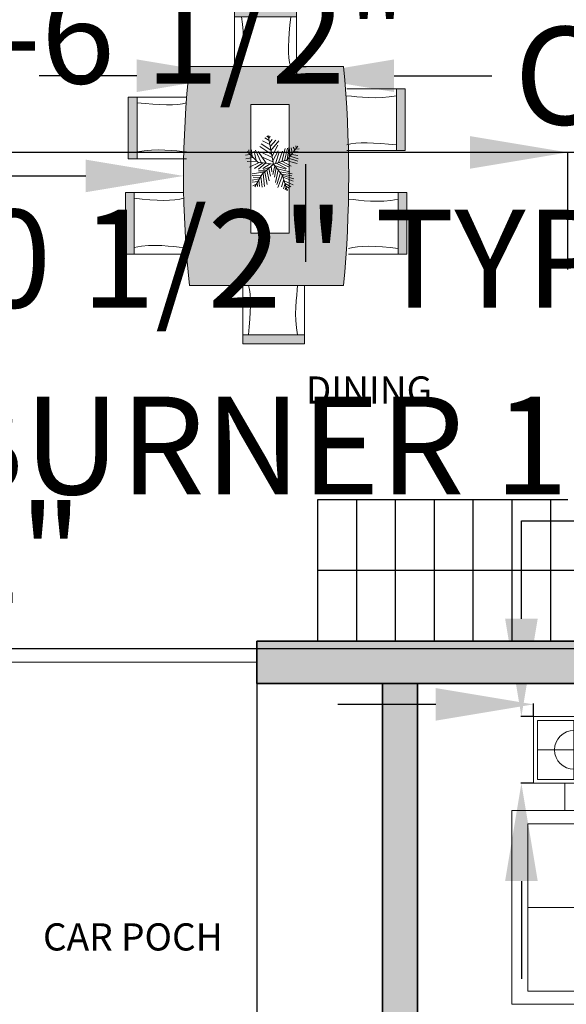
# Model space of a CAD drawing. Units: inches. Extents: x 29 to 6336, y 3 to 2592.
# Tile 5 of 8: x 5531 to 5672, y 2100 to 2354. Entities that reach past the tile are written whole.
import ezdxf

# ---------------------------------------------------------------- set-up
doc = ezdxf.new("R2010")
doc.units = ezdxf.units.IN
doc.header["$MEASUREMENT"] = 0
for name, color, linetype, lineweight in [('A-ANNO-DIMS', 2, 'Continuous', 18), ('A-AREA-IDEN', 7, 'Continuous', 18), ('A-DOOR', 4, 'Continuous', 18), ('A-FLOR-PATT', 9, 'Continuous', 13), ('A-FLOR-STRS', 7, 'Continuous', 25), ('A-FURN', 8, 'Continuous', 18), ('A-FURN-PATT', 18, 'Continuous', 13), ('A-WALL', 7, 'Continuous', 35), ('A-WALL-PATT', 242, 'Continuous', 13), ('L-PLNT', 94, 'Continuous', 18)]:
    doc.layers.add(name, color=color, linetype=linetype, lineweight=lineweight)
doc.styles.get("Standard").update_dxf_attribs({"font": 'arial.ttf'})
doc.dimstyles.get("Standard").update_dxf_attribs({"dimtxt": 25.18, "dimasz": 25.18, "dimexe": 0.18, "dimexo": 0.0625, "dimgap": 0.09, "dimtad": 0, "dimtih": 1, "dimtoh": 1, "dimdec": 0, "dimzin": 0, "dimdsep": 46, "dimlunit": 3, "dimtxsty": 'Standard', "dimcen": 0.09, "dimadec": 0, "dimazin": 0, "dimtfac": 1, "dimtdec": 0, "dimtofl": 0, "dimtmove": 0, "dimatfit": 3, "dimfxl": 1, "dimtolj": 1, "dimtzin": 0, "dimarcsym": 0})

# ---------------------------------------------------------------- blocks, each defined once
blk = doc.blocks.new('*U2')
for p, q in [((-5.114, 28.097), (-24.676, 40.636)), ((-7.288, 39.707), (-21.778, 46.673)), ((-8.737, 47.138), (-17.069, 52.711)), ((-10.186, 53.64), (-13.084, 55.962)), ((0, 0), (-10.5, 57)), ((-9.099, 51.782), (-6.563, 55.962)), ((-7.65, 43.423), (-2.578, 49.46)), ((-5.839, 35.992), (4.667, 48.067)), ((-5.114, 27.632), (10.463, 46.673)), ((-47.498, 19.737), (-55.83, 18.344)), ((-31.5, 4.5), (-52.5, 25.5)), ((-48.585, 21.131), (-49.309, 29.026)), ((-43.513, 28.561), (-42.427, 15.558)), ((-38.442, 26.239), (-34.819, 7.663)), ((-35.544, 28.097), (-24.314, 3.947)), ((-14.533, 2.09), (-30.834, 25.31)), ((-3.665, 19.273), (-27.574, 35.527)), ((-24.314, 23.917), (-2.941, 13.7)), ((-2.941, 16.486), (8.652, 37.85)), ((-1.129, 6.734), (9.014, 26.704)), ((3.942, 1.625), (11.187, 24.381)), ((10.101, 3.483), (17.708, 26.239)), ((16.259, 5.805), (23.142, 31.348)), ((22.055, 7.198), (27.489, 32.277)), ((27, 9), (48, 36)), ((27.127, 9.056), (31.112, 35.992)), ((31.836, 30.883), (32.561, 16.486)), ((35.096, 32.741), (37.27, 22.524)), ((36.183, 19.737), (48.137, 17.88)), ((38.719, 34.134), (41.979, 28.561)), ((40.53, 25.775), (48.862, 24.846)), ((43.791, 29.954), (51.036, 30.883)), ((44.153, 36.456), (45.239, 32.741)), ((-40.615, 13.7), (-55.105, 10.913)), ((-33.37, 6.269), (-52.207, 5.34)), ((-28.299, 3.483), (-47.86, -5.805)), ((-21.416, 3.018), (-38.079, -8.128)), ((0, 0), (-31.5, 4.5)), ((-15.982, 2.09), (-30.11, -9.521)), ((0, 0), (-22.5, -19.5)), ((-6.563, 1.161), (-21.416, -8.128)), ((-20.691, 13.7), (-1.129, 4.876)), ((0, 0), (27, 9)), ((0, 0), (18, -22.5)), ((6.478, 1.625), (26.04, -8.592)), ((11.187, 3.483), (30.749, -5.805)), ((18.07, 5.805), (35.096, -3.483)), ((24.229, 7.663), (46.688, 1.625)), ((29.662, 12.307), (48.137, 6.269)), ((33.285, 16.486), (48.862, 10.913)), ((-17.431, -15.094), (-42.789, -18.809)), ((-22.5, -19.5), (-37.5, -45)), ((-15.257, -12.772), (-30.11, -12.772)), ((-20.691, -18.345), (-17.793, -44.352)), ((-6.563, -5.805), (-19.967, -9.985)), ((-17.069, -15.094), (-12.721, -40.172)), ((-13.446, -11.378), (-8.737, -32.741)), ((-9.461, -8.592), (-6.201, -23.453)), ((-4.752, -3.483), (-3.665, -14.629)), ((2.493, -3.019), (-1.491, -20.202)), ((1.769, -2.555), (24.229, -9.521)), ((5.029, -6.27), (2.131, -25.775)), ((9.014, -11.378), (3.58, -35.992)), ((14.085, -16.951), (6.478, -40.172)), ((7.565, -9.056), (32.198, -14.629)), ((12.274, -15.094), (36.907, -18.809)), ((-28.299, -29.026), (-42.789, -31.348)), ((-24.314, -21.596), (-42.427, -22.06)), ((-30.834, -34.135), (-42.427, -35.528)), ((-26.849, -26.24), (-40.253, -25.775)), ((-32.646, -36.921), (-31.921, -44.352)), ((-29.023, -30.884), (-27.936, -43.887)), ((-25.038, -23.918), (-22.865, -45.281)), ((18.07, -22.524), (8.289, -45.745)), ((20.244, -30.419), (15.897, -44.816)), ((16.259, -19.738), (36.183, -22.989)), ((18, -22.5), (27, -52.5)), ((18.433, -22.524), (40.53, -29.026)), ((19.157, -25.311), (38.719, -33.206)), ((22.78, -37.85), (19.519, -48.532)), ((21.331, -32.741), (39.081, -40.636)), ((22.78, -38.314), (34.372, -44.816)), ((-34.457, -39.708), (-40.978, -42.494)), ((24.591, -45.745), (23.142, -50.854)), ((24.591, -43.423), (30.749, -47.603)), ((26.764, -49.925), (28.213, -50.854))]:
    blk.add_line(p, q)
blk = doc.blocks.new('CHAIR-DINING')
h = blk.add_hatch(color=256)
h.dxf.hatch_style = 1
h.paths.add_polyline_path([(15.9, 12.75), (15.9, 15.02), (0, 15.02), (0, 12.75)])
for p, q in [((0, 0), (0, 15.02)), ((0, 15.02), (15.9, 15.02)), ((0, 12.75), (15.9, 12.75)), ((15.9, 15.02), (15.9, 0))]:
    blk.add_line(p, q)
for points in [[(1.75, 12.75), (2.84, 7.81), (1.97, 2.88), (1.75, 0)], [(14.44, 12.75), (13.78, 7.03), (13.63, 2.52), (14.44, 0)]]:
    blk.add_open_spline(points, degree=3)
blk = doc.blocks.new('SOFA-TWO-SEAT')
blk.add_line((4.12, 24.97), (26.62, 24.97))
for points in [[(4.17, 49.94), (0, 49.94), (0, 0), (4.17, 0)], [(4.17, 49.94), (26.62, 49.94), (26.62, 46.51), (4.17, 46.51)], [(4.17, 3.43), (4.17, 46.51)], [(4.12, 3.43), (26.57, 3.43), (26.57, 0), (4.12, 0)]]:
    blk.add_lwpolyline(points)
blk.add_lwpolyline([(26.62, 46.51), (4.12, 46.51), (4.12, 3.43), (26.62, 3.43)], close=True)
blk = doc.blocks.new('END-TABLE-21X17')
for p, q in [((10.41, 16.21), (10.41, 1)), ((1, 8.6), (19.81, 8.6))]:
    blk.add_line(p, q)
for points in [[(0, 17.21), (20.81, 17.21), (20.81, 0), (0, 0)], [(1, 16.21), (19.81, 16.21), (19.81, 1), (1, 1)]]:
    blk.add_lwpolyline(points, close=True)
blk.add_circle((10.41, 8.6), 5)
blk = doc.blocks.new('*D20')
at = {"layer": 'A-ANNO-DIMS', "color": 0, "lineweight": -2, "transparency": 16777216}
for p, q in [((5586.64, 2341.55), (5586.64, 2339.04)), ((5602.54, 2341.55), (5602.54, 2339.04)), ((5561.46, 2339.22), (5536.28, 2339.22)), ((5627.72, 2339.22), (5652.9, 2339.22))]:
    blk.add_line(p, q, dxfattribs=at)
at = {"layer": 'A-ANNO-DIMS', "color": 0, "transparency": 16777216}
for points in [[(5561.46, 2343.42), (5561.46, 2335.03), (5586.64, 2339.22)], [(5627.72, 2343.42), (5627.72, 2335.03), (5602.54, 2339.22)]]:
    blk.add_solid(points, dxfattribs=at)
at = {"layer": 'Defpoints', "color": 0, "transparency": 16777216}
for p in [(5586.64, 2341.61), (5602.54, 2341.61), (5602.54, 2339.22)]:
    blk.add_point(p, dxfattribs=at)
at = {"layer": 'A-ANNO-DIMS', "color": 0, "transparency": 16777216, "insert": (5789.2, 2339.22), "char_height": 25.18, "attachment_point": 5}
blk.add_mtext('\\A1;CHAIR 1\'-4" TYP.', dxfattribs=at)
blk = doc.blocks.new('*D21')
at = {"layer": 'A-ANNO-DIMS', "color": 0, "lineweight": -2, "transparency": 16777216}
for p, q in [((5604.93, 2381.81), (5604.93, 2406.99)), ((5604.93, 2406.99), (5630.11, 2406.99)), ((5602.6, 2356.63), (5605.11, 2356.63)), ((5602.6, 2341.61), (5605.11, 2341.61)), ((5604.93, 2316.43), (5604.93, 2291.25))]:
    blk.add_line(p, q, dxfattribs=at)
at = {"layer": 'A-ANNO-DIMS', "color": 0, "transparency": 16777216}
for points in [[(5600.73, 2381.81), (5609.12, 2381.81), (5604.93, 2356.63)], [(5600.73, 2316.43), (5609.12, 2316.43), (5604.93, 2341.61)]]:
    blk.add_solid(points, dxfattribs=at)
at = {"layer": 'Defpoints', "color": 0, "transparency": 16777216}
for p in [(5602.54, 2356.63), (5604.93, 2356.63), (5602.54, 2341.61)]:
    blk.add_point(p, dxfattribs=at)
at = {"layer": 'A-ANNO-DIMS', "color": 0, "transparency": 16777216, "insert": (5705.75, 2406.99), "char_height": 25.18, "attachment_point": 5}
blk.add_mtext('\\A1;1\'-3" TYP.', dxfattribs=at)
blk = doc.blocks.new('*D24')
at = {"layer": 'A-ANNO-DIMS', "color": 0, "lineweight": -2, "transparency": 16777216}
for p, q in [((5412.73, 2243.97), (5387.55, 2243.97)), ((5437.91, 2241.81), (5437.91, 2244.15)), ((5452.73, 2241.81), (5452.73, 2244.15)), ((5477.91, 2243.97), (5503.09, 2243.97))]:
    blk.add_line(p, q, dxfattribs=at)
at = {"layer": 'A-ANNO-DIMS', "color": 0, "transparency": 16777216}
for points in [[(5412.73, 2248.16), (5412.73, 2239.77), (5437.91, 2243.97)], [(5477.91, 2248.16), (5477.91, 2239.77), (5452.73, 2243.97)]]:
    blk.add_solid(points, dxfattribs=at)
at = {"layer": 'Defpoints', "color": 0, "transparency": 16777216}
for p in [(5452.73, 2243.97), (5437.91, 2241.74), (5452.73, 2241.74)]:
    blk.add_point(p, dxfattribs=at)
at = {"layer": 'A-ANNO-DIMS', "color": 0, "transparency": 16777216, "insert": (5658.52, 2243.97), "char_height": 25.18, "attachment_point": 5}
blk.add_mtext('\\A1;BURNER 1\'-3" TYP.', dxfattribs=at)
blk = doc.blocks.new('*D25')
at = {"layer": 'A-ANNO-DIMS', "color": 0, "lineweight": -2, "transparency": 16777216}
for p, q in [((5435.68, 2266.92), (5435.68, 2292.1)), ((5435.68, 2292.1), (5460.86, 2292.1)), ((5437.84, 2241.74), (5435.5, 2241.74)), ((5437.84, 2231.12), (5435.5, 2231.12)), ((5435.68, 2205.94), (5435.68, 2180.76))]:
    blk.add_line(p, q, dxfattribs=at)
at = {"layer": 'A-ANNO-DIMS', "color": 0, "transparency": 16777216}
for points in [[(5431.49, 2266.92), (5439.88, 2266.92), (5435.68, 2241.74)], [(5431.49, 2205.94), (5439.88, 2205.94), (5435.68, 2231.12)]]:
    blk.add_solid(points, dxfattribs=at)
at = {"layer": 'Defpoints', "color": 0, "transparency": 16777216}
for p in [(5435.68, 2241.74), (5437.91, 2241.74), (5437.91, 2231.12)]:
    blk.add_point(p, dxfattribs=at)
at = {"layer": 'A-ANNO-DIMS', "color": 0, "transparency": 16777216, "insert": (5576.81, 2292.1), "char_height": 25.18, "attachment_point": 5}
blk.add_mtext('\\A1;0\'-10 1/2" TYP.', dxfattribs=at)
blk = doc.blocks.new('*D28')
at = {"layer": 'A-ANNO-DIMS', "color": 0, "lineweight": -2, "transparency": 16777216}
for p, q in [((5689.81, 2064.89), (5689.81, 2057.28)), ((5739.75, 2064.89), (5739.75, 2057.28)), ((5664.63, 2057.46), (5639.45, 2057.46)), ((5764.93, 2057.46), (5790.11, 2057.46))]:
    blk.add_line(p, q, dxfattribs=at)
at = {"layer": 'A-ANNO-DIMS', "color": 0, "transparency": 16777216}
for points in [[(5664.63, 2061.65), (5664.63, 2053.26), (5689.81, 2057.46)], [(5764.93, 2061.65), (5764.93, 2053.26), (5739.75, 2057.46)]]:
    blk.add_solid(points, dxfattribs=at)
at = {"layer": 'Defpoints', "color": 0, "transparency": 16777216}
for p in [(5689.81, 2064.95), (5739.75, 2064.95), (5689.81, 2057.46)]:
    blk.add_point(p, dxfattribs=at)
at = {"layer": 'A-ANNO-DIMS', "color": 0, "transparency": 16777216, "insert": (5509.91, 2057.46), "char_height": 25.18, "attachment_point": 5}
blk.add_mtext('\\A1;SOFA 4\'-2" TYP.', dxfattribs=at)
blk = doc.blocks.new('*D29')
at = {"layer": 'A-ANNO-DIMS', "color": 0, "lineweight": -2, "transparency": 16777216}
for p, q in [((5682.32, 2116.75), (5682.32, 2141.93)), ((5689.75, 2091.57), (5682.14, 2091.57)), ((5689.75, 2064.95), (5682.14, 2064.95)), ((5682.32, 2039.77), (5682.32, 2014.59))]:
    blk.add_line(p, q, dxfattribs=at)
at = {"layer": 'A-ANNO-DIMS', "color": 0, "transparency": 16777216}
for points in [[(5678.12, 2116.75), (5686.52, 2116.75), (5682.32, 2091.57)], [(5678.12, 2039.77), (5686.52, 2039.77), (5682.32, 2064.95)]]:
    blk.add_solid(points, dxfattribs=at)
at = {"layer": 'Defpoints', "color": 0, "transparency": 16777216}
for p in [(5682.32, 2091.57), (5689.81, 2091.57), (5689.81, 2064.95)]:
    blk.add_point(p, dxfattribs=at)
at = {"layer": 'A-ANNO-DIMS', "color": 0, "transparency": 16777216, "insert": (5682.32, 2078.26), "char_height": 25.18, "attachment_point": 5}
blk.add_mtext('\\A1;2\'-2 1/2" TYP.', dxfattribs=at)
blk = doc.blocks.new('*D34')
at = {"layer": 'A-ANNO-DIMS', "color": 0, "lineweight": -2, "transparency": 16777216}
for p, q in [((5638.44, 2177.3), (5613.26, 2177.3)), ((5663.62, 2174.24), (5663.62, 2177.48)), ((5684.43, 2174.24), (5684.43, 2177.48)), ((5709.61, 2177.3), (5734.79, 2177.3))]:
    blk.add_line(p, q, dxfattribs=at)
at = {"layer": 'A-ANNO-DIMS', "color": 0, "transparency": 16777216}
for points in [[(5638.44, 2181.49), (5638.44, 2173.1), (5663.62, 2177.3)], [(5709.61, 2181.49), (5709.61, 2173.1), (5684.43, 2177.3)]]:
    blk.add_solid(points, dxfattribs=at)
at = {"layer": 'Defpoints', "color": 0, "transparency": 16777216}
for p in [(5684.43, 2177.3), (5663.62, 2174.18), (5684.43, 2174.18)]:
    blk.add_point(p, dxfattribs=at)
at = {"layer": 'A-ANNO-DIMS', "color": 0, "transparency": 16777216, "insert": (5913.59, 2177.3), "char_height": 25.18, "attachment_point": 5}
blk.add_mtext('\\A1;END TABLE 1\'-9" TYP.', dxfattribs=at)
blk = doc.blocks.new('*D35')
at = {"layer": 'A-ANNO-DIMS', "color": 0, "lineweight": -2, "transparency": 16777216}
for p, q in [((5660.5, 2199.36), (5660.5, 2224.54)), ((5660.5, 2224.54), (5685.68, 2224.54)), ((5663.56, 2174.18), (5660.32, 2174.18)), ((5663.56, 2156.97), (5660.32, 2156.97)), ((5660.5, 2131.79), (5660.5, 2106.61))]:
    blk.add_line(p, q, dxfattribs=at)
at = {"layer": 'A-ANNO-DIMS', "color": 0, "transparency": 16777216}
for points in [[(5656.3, 2199.36), (5664.7, 2199.36), (5660.5, 2174.18)], [(5656.3, 2131.79), (5664.7, 2131.79), (5660.5, 2156.97)]]:
    blk.add_solid(points, dxfattribs=at)
at = {"layer": 'Defpoints', "color": 0, "transparency": 16777216}
for p in [(5660.5, 2174.18), (5663.62, 2174.18), (5663.62, 2156.97)]:
    blk.add_point(p, dxfattribs=at)
at = {"layer": 'A-ANNO-DIMS', "color": 0, "transparency": 16777216, "insert": (5761.33, 2224.54), "char_height": 25.18, "attachment_point": 5}
blk.add_mtext('\\A1;1\'-5" TYP.', dxfattribs=at)
blk = doc.blocks.new('*D39')
at = {"layer": 'A-ANNO-DIMS', "color": 0, "lineweight": -2, "transparency": 16777216}
for p, q in [((5417.07, 2045.77), (5417.07, 2070.95)), ((5417.07, 2070.95), (5442.25, 2070.95)), ((5416.29, 2020.59), (5417.25, 2020.59)), ((5416.29, 2015.87), (5417.25, 2015.87)), ((5417.07, 1990.69), (5417.07, 1965.51))]:
    blk.add_line(p, q, dxfattribs=at)
at = {"layer": 'A-ANNO-DIMS', "color": 0, "transparency": 16777216}
for points in [[(5412.88, 2045.77), (5421.27, 2045.77), (5417.07, 2020.59)], [(5412.88, 1990.69), (5421.27, 1990.69), (5417.07, 2015.87)]]:
    blk.add_solid(points, dxfattribs=at)
at = {"layer": 'Defpoints', "color": 0, "transparency": 16777216}
for p in [(5416.23, 2020.59), (5417.07, 2020.59), (5416.23, 2015.87)]:
    blk.add_point(p, dxfattribs=at)
at = {"layer": 'A-ANNO-DIMS', "color": 0, "transparency": 16777216, "insert": (5548.42, 2070.95), "char_height": 25.18, "attachment_point": 5}
blk.add_mtext('\\A1;0\'-4 1/2" TYP.', dxfattribs=at)
blk = doc.blocks.new('*D48')
at = {"layer": 'A-ANNO-DIMS', "color": 0, "lineweight": -2, "transparency": 16777216}
for p, q in [((5351.16, 2319.63), (5351.16, 2522.76)), ((5376.34, 2522.58), (5385.42, 2522.58)), ((5410.6, 2319.63), (5410.6, 2522.76)), ((5410.6, 2522.58), (5435.78, 2522.58))]:
    blk.add_line(p, q, dxfattribs=at)
at = {"layer": 'A-ANNO-DIMS', "color": 0, "transparency": 16777216}
for points in [[(5376.34, 2526.78), (5376.34, 2518.38), (5351.16, 2522.58)], [(5385.42, 2526.78), (5385.42, 2518.38), (5410.6, 2522.58)]]:
    blk.add_solid(points, dxfattribs=at)
at = {"layer": 'Defpoints', "color": 0, "transparency": 16777216}
for p in [(5410.6, 2522.58), (5351.16, 2319.56), (5410.6, 2319.56)]:
    blk.add_point(p, dxfattribs=at)
at = {"layer": 'A-ANNO-DIMS', "color": 0, "transparency": 16777216, "insert": (5508.96, 2522.58), "char_height": 25.18, "attachment_point": 5}
blk.add_mtext('\\A1;4\'-11 1/2"', dxfattribs=at)
blk = doc.blocks.new('*D49')
at = {"layer": 'A-ANNO-DIMS', "color": 0, "lineweight": -2, "transparency": 16777216}
for p, q in [((5419.6, 2191.59), (5419.6, 1921.9)), ((5510.11, 2191.59), (5510.11, 1921.9)), ((5444.78, 1922.08), (5484.93, 1922.08)), ((5510.11, 1922.08), (5535.29, 1922.08))]:
    blk.add_line(p, q, dxfattribs=at)
at = {"layer": 'A-ANNO-DIMS', "color": 0, "transparency": 16777216}
for points in [[(5444.78, 1926.28), (5444.78, 1917.88), (5419.6, 1922.08)], [(5484.93, 1926.28), (5484.93, 1917.88), (5510.11, 1922.08)]]:
    blk.add_solid(points, dxfattribs=at)
at = {"layer": 'Defpoints', "color": 0, "transparency": 16777216}
for p in [(5419.6, 2191.65), (5510.11, 2191.65), (5510.11, 1922.08)]:
    blk.add_point(p, dxfattribs=at)
at = {"layer": 'A-ANNO-DIMS', "color": 0, "transparency": 16777216, "insert": (5598.08, 1922.08), "char_height": 25.18, "attachment_point": 5}
blk.add_mtext('\\A1;7\'-6 1/2"', dxfattribs=at)
blk = doc.blocks.new('*D50')
at = {"layer": 'A-ANNO-DIMS', "color": 0, "lineweight": -2, "transparency": 16777216}
for p, q in [((5510.17, 2319.56), (5917.09, 2319.56)), ((5916.91, 2294.38), (5916.91, 2268.55)), ((5916.91, 2216.83), (5916.91, 2242.66)), ((5510.17, 2191.65), (5917.09, 2191.65))]:
    blk.add_line(p, q, dxfattribs=at)
at = {"layer": 'A-ANNO-DIMS', "color": 0, "transparency": 16777216}
for points in [[(5912.71, 2294.38), (5921.1, 2294.38), (5916.91, 2319.56)], [(5912.71, 2216.83), (5921.1, 2216.83), (5916.91, 2191.65)]]:
    blk.add_solid(points, dxfattribs=at)
at = {"layer": 'Defpoints', "color": 0, "transparency": 16777216}
for p in [(5510.11, 2319.56), (5916.91, 2319.56), (5510.11, 2191.65)]:
    blk.add_point(p, dxfattribs=at)
at = {"layer": 'A-ANNO-DIMS', "color": 0, "transparency": 16777216, "insert": (5916.91, 2255.61), "char_height": 25.18, "attachment_point": 5}
blk.add_mtext('\\A1;10\'-8"', dxfattribs=at)
blk = doc.blocks.new('*D59')
at = {"layer": 'A-ANNO-DIMS', "color": 0, "lineweight": -2, "transparency": 16777216}
for p, q in [((5519.11, 2182.59), (5519.11, 1921.9)), ((5592.36, 2182.59), (5592.36, 1921.9)), ((5493.93, 1922.08), (5468.75, 1922.08)), ((5617.54, 1922.08), (5642.72, 1922.08))]:
    blk.add_line(p, q, dxfattribs=at)
at = {"layer": 'A-ANNO-DIMS', "color": 0, "transparency": 16777216}
for points in [[(5493.93, 1926.28), (5493.93, 1917.88), (5519.11, 1922.08)], [(5617.54, 1926.28), (5617.54, 1917.88), (5592.36, 1922.08)]]:
    blk.add_solid(points, dxfattribs=at)
at = {"layer": 'Defpoints', "color": 0, "transparency": 16777216}
for p in [(5519.11, 2182.65), (5592.36, 2182.65), (5592.36, 1922.08)]:
    blk.add_point(p, dxfattribs=at)
at = {"layer": 'A-ANNO-DIMS', "color": 0, "transparency": 16777216, "insert": (5555.73, 1922.08), "char_height": 25.18, "attachment_point": 5}
blk.add_mtext('\\A1;6\'-1"', dxfattribs=at)
blk = doc.blocks.new('*D60')
at = {"layer": 'A-ANNO-DIMS', "color": 0, "lineweight": -2, "transparency": 16777216}
for p, q in [((5647.28, 2319.47), (5622.1, 2319.47)), ((5672.46, 2289.28), (5672.46, 2319.65)), ((5712.66, 2289.28), (5712.66, 2319.65)), ((5737.84, 2319.47), (5763.02, 2319.47))]:
    blk.add_line(p, q, dxfattribs=at)
at = {"layer": 'A-ANNO-DIMS', "color": 0, "transparency": 16777216}
for points in [[(5647.28, 2323.67), (5647.28, 2315.27), (5672.46, 2319.47)], [(5737.84, 2323.67), (5737.84, 2315.27), (5712.66, 2319.47)]]:
    blk.add_solid(points, dxfattribs=at)
at = {"layer": 'Defpoints', "color": 0, "transparency": 16777216}
for p in [(5712.66, 2319.47), (5672.46, 2289.22), (5712.66, 2289.22)]:
    blk.add_point(p, dxfattribs=at)
at = {"layer": 'A-ANNO-DIMS', "color": 0, "transparency": 16777216, "insert": (5796.57, 2319.47), "char_height": 25.18, "attachment_point": 5}
blk.add_mtext('\\A1;3\'-4"', dxfattribs=at)
blk = doc.blocks.new('*D68')
at = {"layer": 'A-ANNO-DIMS', "color": 0, "lineweight": -2, "transparency": 16777216}
for p, q in [((5479.86, 2259.85), (5479.86, 2285.03)), ((5510.05, 2234.67), (5479.68, 2234.67)), ((5510.05, 2197.33), (5479.68, 2197.33)), ((5479.86, 2172.15), (5479.86, 2146.97))]:
    blk.add_line(p, q, dxfattribs=at)
at = {"layer": 'A-ANNO-DIMS', "color": 0, "transparency": 16777216}
for points in [[(5475.66, 2259.85), (5484.06, 2259.85), (5479.86, 2234.67)], [(5475.66, 2172.15), (5484.06, 2172.15), (5479.86, 2197.33)]]:
    blk.add_solid(points, dxfattribs=at)
at = {"layer": 'Defpoints', "color": 0, "transparency": 16777216}
for p in [(5479.86, 2234.67), (5510.11, 2234.67), (5510.11, 2197.33)]:
    blk.add_point(p, dxfattribs=at)
at = {"layer": 'A-ANNO-DIMS', "color": 0, "transparency": 16777216, "insert": (5479.86, 2216), "char_height": 25.18, "attachment_point": 5}
blk.add_mtext('\\A1;3\'-1 1/2"', dxfattribs=at)
blk = doc.blocks.new('*D69')
at = {"layer": 'A-ANNO-DIMS', "color": 0, "lineweight": -2, "transparency": 16777216}
for p, q in [((5394.42, 2349.81), (5369.24, 2349.81)), ((5419.6, 2319.63), (5419.6, 2349.99)), ((5450.34, 2319.63), (5450.34, 2349.99)), ((5475.52, 2349.81), (5500.7, 2349.81))]:
    blk.add_line(p, q, dxfattribs=at)
at = {"layer": 'A-ANNO-DIMS', "color": 0, "transparency": 16777216}
for points in [[(5394.42, 2354.01), (5394.42, 2345.62), (5419.6, 2349.81)], [(5475.52, 2354.01), (5475.52, 2345.62), (5450.34, 2349.81)]]:
    blk.add_solid(points, dxfattribs=at)
at = {"layer": 'Defpoints', "color": 0, "transparency": 16777216}
for p in [(5450.34, 2349.81), (5419.6, 2319.56), (5450.34, 2319.56)]:
    blk.add_point(p, dxfattribs=at)
at = {"layer": 'A-ANNO-DIMS', "color": 0, "transparency": 16777216, "insert": (5563.81, 2349.81), "char_height": 25.18, "attachment_point": 5}
blk.add_mtext('\\A1;2\'-6 1/2"', dxfattribs=at)
blk = doc.blocks.new('*D71')
at = {"layer": 'A-ANNO-DIMS', "color": 0, "lineweight": -2, "transparency": 16777216}
for p, q in [((5510.6, 2313.41), (5548.31, 2313.41)), ((5835.74, 2313.41), (5835.92, 2313.41)), ((5835.83, 2313.32), (5835.83, 2313.5))]:
    blk.add_line(p, q, dxfattribs=at)
at = {"layer": 'A-ANNO-DIMS', "color": 0, "transparency": 16777216}
blk.add_solid([(5548.31, 2317.61), (5548.31, 2309.22), (5573.49, 2313.41)], dxfattribs=at)
at = {"layer": 'Defpoints', "color": 0, "transparency": 16777216}
for p in [(5573.49, 2313.41), (5835.83, 2313.41)]:
    blk.add_point(p, dxfattribs=at)
at = {"layer": 'A-ANNO-DIMS', "color": 0, "transparency": 16777216, "insert": (5416.09, 2313.41), "char_height": 25.18, "attachment_point": 5}
blk.add_mtext('\\A1;R21\'-10 1/2"', dxfattribs=at)

msp = doc.modelspace()

# ---------------------------------------------------------------- hatches: boundary and pattern name
at = {"layer": 'A-FURN-PATT'}
h = msp.add_hatch(color=256, dxfattribs=at)
h.dxf.hatch_style = 1
h.paths.add_polyline_path([(5614.72, 2341.61), (5575.01, 2341.61, 0.053894), (5575.01, 2285.22), (5614.72, 2285.22, 0.046017)])
h.paths.add_polyline_path([(5590.82, 2298.69), (5590.82, 2331.84), (5600.65, 2331.84), (5600.65, 2318.19), (5600.89, 2318.49), (5600.88, 2318.57), (5600.93, 2318.55), (5600.65, 2318.19), (5600.65, 2298.69)], flags=16)
h.paths.add_polyline_path([(5599.61, 2311.45), (5599.6, 2311.44), (5599.61, 2311.43)], flags=0)
h.paths.add_polyline_path([(5599.01, 2313.47), (5596.67, 2316.4), (5594.45, 2314.47), (5594.45, 2314.45), (5594.41, 2314.44), (5596.67, 2316.4), (5595.99, 2320.04), (5596.04, 2320.02), (5596.01, 2319.98), (5596.67, 2316.4), (5596.94, 2316.05), (5597, 2316.03), (5596.99, 2316), (5598.98, 2313.5), (5599.01, 2313.49)], flags=0)
at = {"layer": 'A-WALL-PATT'}
h = msp.add_hatch(color=256, dxfattribs=at)
h.dxf.hatch_style = 1
h.paths.add_polyline_path([(5558.68, 2492.33), (5459.71, 2492.33), (5459.71, 2483.33), (5511.77, 2483.33), (5511.77, 2388.68), (5520.77, 2388.68), (5520.77, 2393.05), (5526.31, 2393.05), (5526.31, 2402.05), (5520.77, 2402.05), (5520.77, 2483.33), (5558.68, 2483.33)])
h.paths.add_polyline_path([(5659.13, 2492.33), (5586.68, 2492.33), (5586.68, 2483.33), (5624.6, 2483.33), (5624.6, 2402.05), (5562.29, 2402.05), (5562.29, 2393.05), (5676.48, 2393.05), (5676.48, 2402.05), (5633.6, 2402.05), (5633.6, 2422.71), (5633.6, 2483.33), (5659.13, 2483.33)])
h.paths.add_polyline_path([(5886.66, 2492.33), (5687.13, 2492.33), (5687.13, 2483.33), (5712.66, 2483.33), (5712.66, 2468.69), (5721.66, 2468.69), (5721.66, 2483.33), (5877.66, 2483.33), (5877.66, 2106.48), (5858.21, 2106.48), (5858.21, 2097.48), (5877.66, 2097.48), (5877.66, 1961.33), (5877.66, 1952.33), (5886.66, 1952.33)])
h.paths.add_polyline_path([(5721.66, 2416.69), (5712.66, 2416.69), (5712.66, 2402.05), (5709.45, 2402.05), (5709.45, 2393.05), (5712.66, 2393.05), (5712.66, 2386.01), (5721.66, 2386.01)], flags=17)
h.paths.add_polyline_path([(5355.66, 2483.33), (5407.71, 2483.33), (5407.71, 2492.33), (5346.66, 2492.33), (5346.66, 2431.95), (5355.66, 2431.95)])
h.paths.add_polyline_path([(5355.66, 2379.95), (5346.66, 2379.95), (5346.66, 2319.56), (5355.66, 2319.56), (5355.66, 2328.56)])
h.paths.add_polyline_path([(5520.77, 2337.13), (5511.77, 2337.13), (5511.77, 2328.56), (5410.6, 2328.56), (5410.6, 2319.56), (5410.6, 2281.61), (5419.6, 2281.61), (5419.6, 2319.56), (5510.11, 2319.56), (5510.11, 2234.67), (5519.11, 2234.67), (5519.11, 2319.56), (5520.77, 2319.56)])
h.paths.add_polyline_path([(5519.11, 2197.33), (5510.11, 2197.33), (5510.11, 2191.65), (5419.6, 2191.65), (5419.6, 2228.6), (5419.6, 2229.61), (5410.6, 2229.61), (5410.6, 2182.65), (5519.11, 2182.65)])
h.paths.add_polyline_path([(5712.66, 2193.6), (5592.36, 2193.6), (5592.36, 2182.65), (5624.77, 2182.65), (5633.77, 2182.65), (5712.66, 2182.65)])
h.paths.add_polyline_path([(5633.77, 2182.65), (5624.77, 2182.65), (5624.77, 2051.72), (5633.77, 2051.72), (5691.77, 2051.72), (5691.77, 2060.72), (5633.77, 2060.72)])
h.paths.add_polyline_path([(5810.76, 2097.48), (5830.21, 2097.48), (5830.21, 2106.48), (5810.76, 2106.48), (5810.76, 2182.65), (5817.87, 2182.65), (5817.87, 2193.6), (5783.59, 2193.6), (5783.59, 2182.65), (5801.76, 2182.65), (5801.76, 2060.72), (5743.77, 2060.72), (5743.77, 2051.72), (5810.76, 2051.72)], flags=17)
h.paths.add_polyline_path([(5721.66, 2319.56), (5877.66, 2319.56), (5877.66, 2328.56), (5721.66, 2328.56), (5721.66, 2335.85), (5712.66, 2335.85), (5712.66, 2319.56), (5712.66, 2182.65), (5726.12, 2182.65), (5726.12, 2193.6), (5721.66, 2193.6)], flags=17)
h.paths.add_polyline_path([(5631.73, 2431.78), (5711.31, 2431.78), (5711.31, 2446.2), (5631.73, 2446.2)], flags=9)

# ---------------------------------------------------------------- linework, layer by layer
at = {"layer": 'A-DOOR'}
msp.add_line((5592.36, 2188.13), (5519.11, 2188.13), dxfattribs=at)
at = {"layer": 'A-FLOR-PATT'}
msp.add_line((5671.67, 2156.97), (5671.67, 2149.97), dxfattribs=at)
at = {"layer": 'A-FLOR-STRS'}
for p, q in [((5608.08, 2193.6), (5608.08, 2230.08)), ((5608.08, 2230.08), (5672.46, 2230.08)), ((5618.08, 2193.6), (5618.08, 2230.08)), ((5628.08, 2193.6), (5628.08, 2230.08)), ((5638.08, 2193.6), (5638.08, 2230.08)), ((5648.08, 2193.6), (5648.08, 2230.08)), ((5658.08, 2193.6), (5658.08, 2230.08)), ((5668.08, 2193.6), (5668.08, 2230.08)), ((5608.08, 2211.84), (5693.88, 2211.84))]:
    msp.add_line(p, q, dxfattribs=at)
at = {"layer": 'A-FURN'}
for points in [[(5575.01, 2341.61), (5614.72, 2341.61)], [(5614.72, 2285.22), (5614.72, 2285.22), (5575.01, 2285.22)]]:
    msp.add_lwpolyline(points, dxfattribs=at)
msp.add_lwpolyline([(5590.82, 2331.84), (5600.65, 2331.84), (5600.65, 2298.69), (5590.82, 2298.69)], close=True, dxfattribs=at)
for centre, radius, start, end in [((5835.83, 2313.41), 262.34, 173.8302, 186.1698), ((5309.02, 2313.41), 307, 354.7306, 5.2694)]:
    msp.add_arc(centre, radius, start, end, dxfattribs=at)
at = {"layer": 'A-WALL'}
for p, q in [((5592.36, 2193.6), (5712.66, 2193.6)), ((5592.36, 2193.6), (5592.36, 2182.65)), ((5592.36, 2182.65), (5624.77, 2182.65)), ((5624.77, 2182.65), (5624.77, 2051.72)), ((5624.77, 2182.65), (5633.77, 2182.65)), ((5633.77, 2182.65), (5633.77, 2060.72)), ((5633.77, 2182.65), (5712.66, 2182.65))]:
    msp.add_line(p, q, dxfattribs=at)

# ---------------------------------------------------------------- block references
at = {"layer": 'A-FURN'}
for name, p in [('CHAIR-DINING', (5586.64, 2341.61)), ('END-TABLE-21X17', (5663.62, 2156.97)), ('SOFA-TWO-SEAT', (5658, 2100.03))]:
    msp.add_blockref(name, p, dxfattribs=at)
for p, rotation in [((5574.28, 2317.84), 90.00000000001506), ((5615.57, 2335.82), 270.0000000000055), ((5573.53, 2293.22), 90.00000000000794), ((5616.01, 2309.17), 270.000000000008), ((5604.62, 2285.22), 180)]:
    msp.add_blockref('CHAIR-DINING', p, dxfattribs=dict(at, rotation=rotation))
at = {"layer": 'L-PLNT', "xscale": 0.129609211949132, "yscale": 0.129609211949132, "zscale": 0.129609211949132}
msp.add_blockref('*U2', (5596.67, 2316.4), dxfattribs=at)

# ---------------------------------------------------------------- texts
at = {"layer": 'A-AREA-IDEN', "char_height": 7, "attachment_point": 1}
for s, insert in [('DINING', (5604.97, 2261.77)), ('CAR POCH', (5537.29, 2120.89))]:
    msp.add_mtext_dynamic_manual_height_columns(s, width=54.3344, gutter_width=1, heights=[0], dxfattribs=dict(at, insert=insert))

# ---------------------------------------------------------------- dimensions: what is measured, and where the dimension line sits
at = {"layer": 'A-ANNO-DIMS'}
for base, p1, p2, picture, middle in [((5410.6, 2522.58), (5351.16, 2319.56), (5410.6, 2319.56), '*D48', (5508.96, 2522.58)), ((5450.34, 2349.81), (5419.6, 2319.56), (5450.34, 2319.56), '*D69', (5563.81, 2349.81)), ((5712.66, 2319.47), (5672.46, 2289.22), (5712.66, 2289.22), '*D60', (5796.57, 2319.47)), ((5510.11, 1922.08), (5419.6, 2191.65), (5510.11, 2191.65), '*D49', (5598.08, 1922.08)), ((5592.3592, 1922.0797), (5519.1102, 2182.6481), (5592.3592, 2182.6517), '*D59', (5555.7347, 1922.0797))]:
    dim = msp.add_linear_dim(base=base, p1=p1, p2=p2, dimstyle='Standard', override={"dimdec": 1, "dimlfac": 1, "dimrnd": 0, "dimzin": 1, "dimdsep": 46, "dimlunit": 4, "dimfrac": 2}, dxfattribs=at)
    dim.commit()
    dim.dimension.update_dxf_attribs({"geometry": picture, "text_midpoint": middle})
for base, p1, p2, angle, text, picture, middle in [((5604.93, 2356.63), (5602.54, 2341.61), (5602.54, 2356.63), 90, '<> TYP.', '*D21', (5705.75, 2406.99)), ((5435.68, 2241.74), (5437.91, 2231.12), (5437.91, 2241.74), 90, '<> TYP.', '*D25', (5576.81, 2292.1)), ((5660.5, 2174.18), (5663.62, 2156.97), (5663.62, 2174.18), 90, '<> TYP.', '*D35', (5761.33, 2224.54)), ((5682.32, 2091.57), (5689.81, 2064.95), (5689.81, 2091.57), 90, '<> TYP.', '*D29', (5682.32, 2078.26)), ((5417.07, 2020.59), (5416.23, 2015.87), (5416.23, 2020.59), 90, '<> TYP.', '*D39', (5548.42, 2070.95)), ((5689.81, 2057.46), (5739.75, 2064.95), (5689.81, 2064.95), 180, 'SOFA <> TYP.', '*D28', (5509.91, 2057.46))]:
    dim = msp.add_linear_dim(base=base, p1=p1, p2=p2, angle=angle, text=text, dimstyle='Standard', override={"dimdec": 1, "dimlfac": 1, "dimrnd": 0, "dimzin": 1, "dimdsep": 46, "dimlunit": 4, "dimfrac": 2}, dxfattribs=at)
    dim.commit()
    dim.dimension.update_dxf_attribs({"geometry": picture, "text_midpoint": middle})
for base, p1, p2, text, picture, middle in [((5602.54, 2339.22), (5586.64, 2341.61), (5602.54, 2341.61), 'CHAIR <> TYP.', '*D20', (5789.2, 2339.22)), ((5452.73, 2243.97), (5437.91, 2241.74), (5452.73, 2241.74), 'BURNER <> TYP.', '*D24', (5658.52, 2243.97)), ((5684.43, 2177.3), (5663.62, 2174.18), (5684.43, 2174.18), 'END TABLE <> TYP.', '*D34', (5913.59, 2177.3))]:
    dim = msp.add_linear_dim(base=base, p1=p1, p2=p2, text=text, dimstyle='Standard', override={"dimdec": 1, "dimlfac": 1, "dimrnd": 0, "dimzin": 1, "dimdsep": 46, "dimlunit": 4, "dimfrac": 2}, dxfattribs=at)
    dim.commit()
    dim.dimension.update_dxf_attribs({"geometry": picture, "text_midpoint": middle})
dim = msp.add_radius_dim(center=(5835.83, 2313.41), mpoint=(5573.49, 2313.41), dimstyle='Standard', override={"dimdec": 1, "dimlfac": 1, "dimrnd": 0, "dimzin": 1, "dimdsep": 46, "dimlunit": 4, "dimfrac": 2}, dxfattribs=at)
dim.commit()
dim.dimension.update_dxf_attribs({"geometry": '*D71', "text_midpoint": (5416.09, 2313.41), "dimtype": 164})
for base, p1, p2, picture, middle in [((5916.91, 2319.56), (5510.11, 2191.65), (5510.11, 2319.56), '*D50', (5916.91, 2255.61)), ((5479.86, 2234.67), (5510.11, 2197.33), (5510.11, 2234.67), '*D68', (5479.86, 2216))]:
    dim = msp.add_linear_dim(base=base, p1=p1, p2=p2, angle=90, dimstyle='Standard', override={"dimdec": 1, "dimlfac": 1, "dimrnd": 0, "dimzin": 1, "dimdsep": 46, "dimlunit": 4, "dimfrac": 2}, dxfattribs=at)
    dim.commit()
    dim.dimension.update_dxf_attribs({"geometry": picture, "text_midpoint": middle})

doc.saveas('drawing.dxf')
